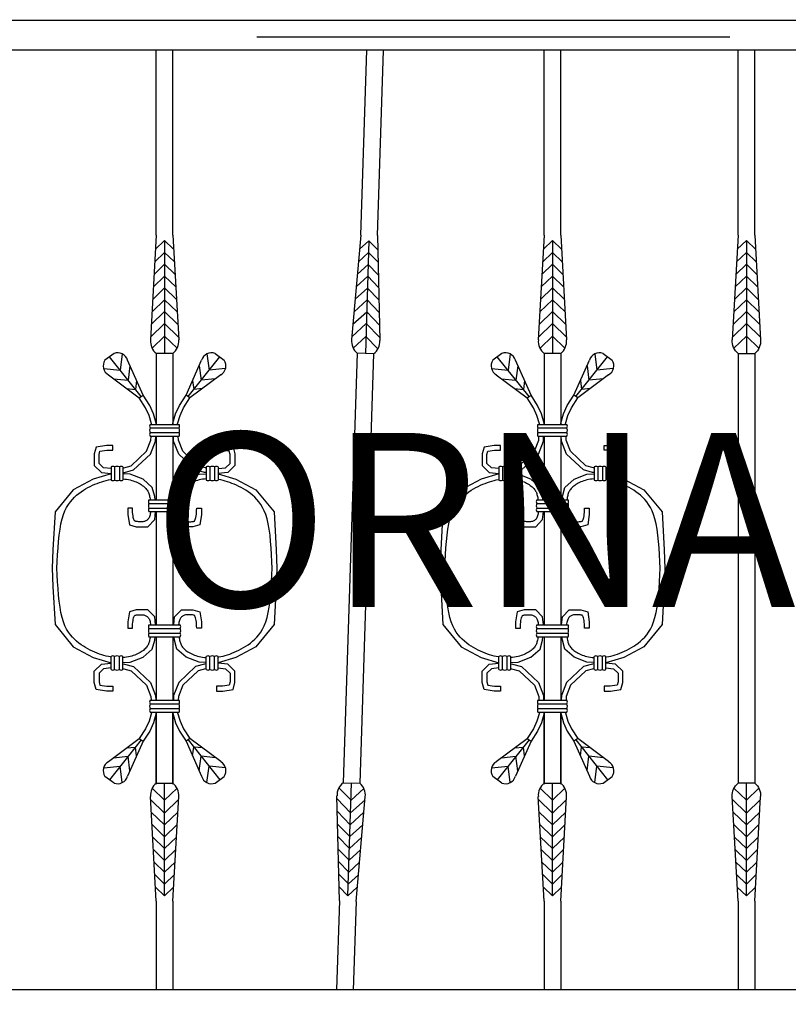
# Model space of a CAD drawing. Units: inches. Extents: x 2278 to 7495, y -71 to 1198.
# Tile 21 of 44: x 5033 to 5060, y 126 to 160. Entities that reach past the tile are written whole.
import ezdxf

# ---------------------------------------------------------------- set-up
doc = ezdxf.new("R2010")
doc.units = ezdxf.units.IN
doc.header["$MEASUREMENT"] = 0
doc.layers.add('A-ANNO-DIMS', color=2, linetype='Continuous', lineweight=18)
doc.layers.add('A-ELEV', color=7, linetype='Continuous', lineweight=25)
doc.styles.get("Standard").update_dxf_attribs({"font": 'arial.ttf'})
doc.dimstyles.get("Standard").update_dxf_attribs({"dimtxt": 6, "dimasz": 3, "dimexe": 0.18, "dimexo": 0.0625, "dimgap": 0.09, "dimtad": 0, "dimtih": 1, "dimtoh": 1, "dimdec": 0, "dimzin": 0, "dimdsep": 46, "dimlunit": 3, "dimtxsty": 'Standard', "dimblk": 'ARCHTICK', "dimcen": 0.09, "dimadec": 0, "dimazin": 0, "dimtfac": 1, "dimtdec": 0, "dimtofl": 0, "dimtmove": 0, "dimatfit": 3, "dimfxl": 1, "dimtolj": 1, "dimtzin": 0, "dimarcsym": 0})

# ---------------------------------------------------------------- blocks, each defined once
blk = doc.blocks.new('BALUSTER-ORNATE-A')
for p, q in [((3.585, 26.003), (3.585, 32.384)), ((4.155, 26.003), (4.155, 32.38)), ((3.585, 26.003), (3.383, 22.393)), ((3.558, 25.516), (3.87, 25.818)), ((3.87, 25.818), (3.87, 21.929)), ((4.182, 25.516), (3.87, 25.818)), ((4.155, 26.003), (4.357, 22.393)), ((3.533, 25.084), (3.87, 25.41)), ((4.207, 25.084), (3.87, 25.41)), ((3.509, 24.653), (3.87, 25.001)), ((4.231, 24.653), (3.87, 25.001)), ((3.485, 24.221), (3.87, 24.593)), ((4.255, 24.221), (3.87, 24.593)), ((3.461, 23.79), (3.87, 24.185)), ((4.279, 23.79), (3.87, 24.185)), ((3.437, 23.358), (3.87, 23.777)), ((4.303, 23.358), (3.87, 23.777)), ((3.413, 22.927), (3.87, 23.369)), ((4.327, 22.927), (3.87, 23.369)), ((3.388, 22.495), (3.87, 22.961)), ((4.352, 22.495), (3.87, 22.961)), ((3.442, 22.106), (3.87, 22.52)), ((4.299, 22.106), (3.87, 22.52)), ((2.128, 21.929), (1.813, 21.699)), ((3.063, 20.442), (1.97, 21.814)), ((2.412, 21.914), (2.339, 21.352)), ((3.585, 21.929), (3.585, 19.485)), ((4.155, 21.929), (3.585, 21.929)), ((4.155, 21.929), (4.155, 19.485)), ((4.677, 20.442), (5.77, 21.814)), ((5.328, 21.914), (5.401, 21.352)), ((5.612, 21.929), (5.927, 21.699)), ((1.774, 21.406), (2.339, 21.352)), ((3.131, 20.487), (2.594, 21.696)), ((2.678, 21.507), (2.613, 21.007)), ((4.609, 20.487), (5.146, 21.696)), ((5.062, 21.507), (5.127, 21.007)), ((5.966, 21.406), (5.401, 21.352)), ((1.936, 21.192), (2.995, 20.398)), ((2.111, 21.055), (2.613, 21.007)), ((5.804, 21.192), (4.745, 20.398)), ((5.629, 21.055), (5.127, 21.007)), ((2.562, 20.717), (2.868, 20.688)), ((2.907, 20.992), (2.868, 20.688)), ((4.833, 20.992), (4.872, 20.688)), ((5.178, 20.717), (4.872, 20.688)), ((2.995, 20.398), (3.131, 20.487)), ((3.217, 20.057), (2.995, 20.398)), ((3.36, 20.135), (3.131, 20.487)), ((4.38, 20.135), (4.609, 20.487)), ((4.523, 20.057), (4.745, 20.398)), ((4.745, 20.398), (4.609, 20.487)), ((3.337, 19.795), (3.217, 20.057)), ((3.49, 19.852), (3.36, 20.135)), ((4.25, 19.852), (4.38, 20.135)), ((4.403, 19.795), (4.523, 20.057)), ((3.421, 19.506), (3.337, 19.795)), ((3.585, 19.526), (3.49, 19.852)), ((4.155, 19.526), (4.25, 19.852)), ((4.319, 19.506), (4.403, 19.795)), ((3.37, 19.485), (4.37, 19.485)), ((3.37, 19.363), (4.37, 19.363)), ((3.42, 19.485), (3.421, 19.506)), ((3.583, 19.485), (3.585, 19.526)), ((4.157, 19.485), (4.155, 19.526)), ((4.32, 19.485), (4.319, 19.506)), ((3.37, 19.2), (4.37, 19.2)), ((3.37, 19.077), (4.37, 19.077)), ((3.396, 18.942), (3.402, 19.077)), ((3.558, 18.908), (3.565, 19.077)), ((3.585, 19.077), (3.585, 16.887)), ((4.155, 19.077), (4.155, 16.887)), ((4.182, 18.908), (4.175, 19.077)), ((4.344, 18.942), (4.338, 19.077)), ((1.513, 18.705), (1.449, 18.469)), ((1.866, 18.759), (1.513, 18.705)), ((2.084, 18.759), (1.866, 18.759)), ((2.084, 18.596), (2.084, 18.759)), ((3.247, 18.557), (3.396, 18.942)), ((3.385, 18.463), (3.558, 18.908)), ((4.355, 18.463), (4.182, 18.908)), ((4.493, 18.557), (4.344, 18.942)), ((5.656, 18.596), (5.656, 18.759)), ((5.656, 18.759), (5.874, 18.759)), ((5.874, 18.759), (6.227, 18.705)), ((6.227, 18.705), (6.291, 18.469)), ((1.449, 18.469), (1.449, 18.069)), ((1.612, 18.447), (1.642, 18.56)), ((1.612, 18.138), (1.612, 18.447)), ((1.642, 18.56), (1.879, 18.596)), ((1.879, 18.596), (2.084, 18.596)), ((2.719, 18.062), (3.247, 18.557)), ((2.801, 17.915), (3.385, 18.463)), ((4.939, 17.915), (4.355, 18.463)), ((5.021, 18.062), (4.493, 18.557)), ((5.861, 18.596), (5.656, 18.596)), ((6.098, 18.56), (5.861, 18.596)), ((6.128, 18.447), (6.098, 18.56)), ((6.128, 18.138), (6.128, 18.447)), ((6.291, 18.469), (6.291, 18.069)), ((1.449, 18.069), (1.694, 17.833)), ((1.767, 17.989), (1.612, 18.138)), ((2.026, 17.961), (1.767, 17.989)), ((2.026, 18.021), (2.026, 17.565)), ((2.148, 18.021), (2.148, 17.565)), ((2.311, 18.021), (2.311, 17.565)), ((2.434, 18.021), (2.434, 17.565)), ((2.434, 17.99), (2.462, 17.993)), ((2.462, 17.993), (2.719, 18.062)), ((5.278, 17.993), (5.021, 18.062)), ((5.306, 17.99), (5.278, 17.993)), ((5.306, 18.021), (5.306, 17.565)), ((5.429, 18.021), (5.429, 17.565)), ((5.592, 18.021), (5.592, 17.565)), ((5.714, 18.021), (5.714, 17.565)), ((5.714, 17.961), (5.973, 17.989)), ((5.973, 17.989), (6.128, 18.138)), ((6.291, 18.069), (6.046, 17.833)), ((2.026, 17.782), (1.412, 17.603)), ((1.694, 17.833), (2.026, 17.797)), ((2.434, 17.826), (2.492, 17.833)), ((2.683, 17.766), (2.434, 17.777)), ((2.492, 17.833), (2.801, 17.915)), ((3.128, 17.594), (2.683, 17.766)), ((4.612, 17.594), (5.057, 17.766)), ((5.248, 17.833), (4.939, 17.915)), ((5.057, 17.766), (5.306, 17.777)), ((5.306, 17.826), (5.248, 17.833)), ((6.046, 17.833), (5.714, 17.797)), ((5.714, 17.782), (6.328, 17.603)), ((1.412, 17.603), (0.722, 17.231)), ((1.15, 17.265), (1.23, 17.309)), ((1.23, 17.309), (1.309, 17.35)), ((1.309, 17.35), (1.389, 17.388)), ((1.389, 17.388), (1.469, 17.422)), ((1.469, 17.422), (1.549, 17.454)), ((1.549, 17.454), (1.627, 17.484)), ((1.627, 17.484), (1.705, 17.51)), ((1.705, 17.51), (1.782, 17.533)), ((1.782, 17.533), (1.858, 17.553)), ((1.858, 17.553), (1.933, 17.571)), ((1.933, 17.571), (2.007, 17.585)), ((2.007, 17.585), (2.026, 17.587)), ((2.434, 17.606), (2.499, 17.6)), ((2.499, 17.6), (2.563, 17.592)), ((2.563, 17.592), (2.624, 17.582)), ((2.624, 17.582), (2.683, 17.57)), ((2.683, 17.57), (2.739, 17.556)), ((2.739, 17.556), (2.792, 17.54)), ((2.792, 17.54), (2.843, 17.522)), ((2.843, 17.522), (2.891, 17.503)), ((2.891, 17.503), (2.937, 17.482)), ((2.937, 17.482), (2.981, 17.46)), ((2.981, 17.46), (3.024, 17.436)), ((3.024, 17.436), (3.064, 17.41)), ((3.064, 17.41), (3.102, 17.384)), ((3.102, 17.384), (3.138, 17.357)), ((3.446, 17.313), (3.128, 17.594)), ((3.138, 17.357), (3.171, 17.329)), ((3.171, 17.329), (3.201, 17.301)), ((3.201, 17.301), (3.228, 17.272)), ((3.528, 17.004), (3.446, 17.313)), ((4.212, 17.004), (4.294, 17.313)), ((4.294, 17.313), (4.612, 17.594)), ((4.539, 17.301), (4.512, 17.272)), ((4.569, 17.329), (4.539, 17.301)), ((4.602, 17.357), (4.569, 17.329)), ((4.638, 17.384), (4.602, 17.357)), ((4.676, 17.41), (4.638, 17.384)), ((4.716, 17.436), (4.676, 17.41)), ((4.759, 17.46), (4.716, 17.436)), ((4.803, 17.482), (4.759, 17.46)), ((4.849, 17.503), (4.803, 17.482)), ((4.897, 17.522), (4.849, 17.503)), ((4.948, 17.54), (4.897, 17.522)), ((5.001, 17.556), (4.948, 17.54)), ((5.057, 17.57), (5.001, 17.556)), ((5.116, 17.582), (5.057, 17.57)), ((5.177, 17.592), (5.116, 17.582)), ((5.241, 17.6), (5.177, 17.592)), ((5.306, 17.606), (5.241, 17.6)), ((5.733, 17.585), (5.714, 17.587)), ((5.807, 17.571), (5.733, 17.585)), ((5.882, 17.553), (5.807, 17.571)), ((5.958, 17.533), (5.882, 17.553)), ((6.035, 17.51), (5.958, 17.533)), ((6.113, 17.484), (6.035, 17.51)), ((6.191, 17.454), (6.113, 17.484)), ((6.271, 17.422), (6.191, 17.454)), ((6.351, 17.388), (6.271, 17.422)), ((6.328, 17.603), (7.018, 17.231)), ((6.431, 17.35), (6.351, 17.388)), ((6.51, 17.309), (6.431, 17.35)), ((6.59, 17.265), (6.51, 17.309)), ((0.722, 17.231), (0.096, 16.469)), ((0.692, 16.9), (0.764, 16.975)), ((0.764, 16.975), (0.839, 17.043)), ((0.839, 17.043), (0.916, 17.105)), ((0.916, 17.105), (0.993, 17.163)), ((0.993, 17.163), (1.071, 17.216)), ((1.071, 17.216), (1.15, 17.265)), ((3.228, 17.272), (3.252, 17.244)), ((3.252, 17.244), (3.272, 17.217)), ((3.272, 17.217), (3.288, 17.19)), ((3.288, 17.19), (3.303, 17.162)), ((3.303, 17.162), (3.316, 17.134)), ((3.316, 17.134), (3.327, 17.104)), ((3.327, 17.104), (3.337, 17.072)), ((3.337, 17.072), (3.346, 17.038)), ((3.346, 17.038), (3.354, 17.001)), ((3.354, 17.001), (3.361, 16.962)), ((3.361, 16.962), (3.368, 16.922)), ((3.542, 16.887), (3.528, 17.004)), ((4.198, 16.887), (4.212, 17.004)), ((4.379, 16.962), (4.372, 16.922)), ((4.386, 17.001), (4.379, 16.962)), ((4.394, 17.038), (4.386, 17.001)), ((4.403, 17.072), (4.394, 17.038)), ((4.413, 17.104), (4.403, 17.072)), ((4.424, 17.134), (4.413, 17.104)), ((4.437, 17.162), (4.424, 17.134)), ((4.452, 17.19), (4.437, 17.162)), ((4.468, 17.217), (4.452, 17.19)), ((4.489, 17.244), (4.468, 17.217)), ((4.512, 17.272), (4.489, 17.244)), ((6.669, 17.216), (6.59, 17.265)), ((6.747, 17.163), (6.669, 17.216)), ((6.824, 17.105), (6.747, 17.163)), ((6.901, 17.043), (6.824, 17.105)), ((6.976, 16.975), (6.901, 17.043)), ((7.048, 16.9), (6.976, 16.975)), ((7.018, 17.231), (7.644, 16.469)), ((0.438, 16.508), (0.495, 16.624)), ((0.495, 16.624), (0.557, 16.727)), ((0.557, 16.727), (0.623, 16.819)), ((0.623, 16.819), (0.692, 16.9)), ((3.329, 16.887), (4.411, 16.887)), ((3.329, 16.764), (4.411, 16.764)), ((3.368, 16.922), (3.374, 16.887)), ((4.372, 16.922), (4.366, 16.887)), ((7.117, 16.819), (7.048, 16.9)), ((7.183, 16.727), (7.117, 16.819)), ((7.245, 16.624), (7.183, 16.727)), ((7.302, 16.508), (7.245, 16.624)), ((0.096, 16.469), (0.025, 15.162)), ((0.34, 16.227), (0.386, 16.376)), ((0.386, 16.376), (0.438, 16.508)), ((2.764, 16.599), (2.602, 16.596)), ((2.602, 16.596), (2.602, 16.378)), ((2.602, 16.378), (2.656, 16.024)), ((2.766, 16.522), (2.764, 16.599)), ((2.769, 16.452), (2.766, 16.522)), ((2.775, 16.388), (2.769, 16.452)), ((2.783, 16.331), (2.775, 16.388)), ((2.792, 16.28), (2.783, 16.331)), ((3.329, 16.601), (4.411, 16.601)), ((3.329, 16.479), (4.411, 16.479)), ((3.346, 16.299), (3.333, 16.271)), ((3.357, 16.329), (3.346, 16.299)), ((3.368, 16.364), (3.357, 16.329)), ((3.376, 16.401), (3.368, 16.364)), ((3.383, 16.441), (3.376, 16.401)), ((3.388, 16.479), (3.383, 16.441)), ((3.528, 16.206), (3.557, 16.479)), ((3.585, 16.479), (3.585, 12.578)), ((4.155, 16.479), (4.155, 12.578)), ((4.212, 16.206), (4.183, 16.479)), ((4.352, 16.479), (4.357, 16.441)), ((4.357, 16.441), (4.364, 16.401)), ((4.364, 16.401), (4.372, 16.364)), ((4.372, 16.364), (4.383, 16.329)), ((4.383, 16.329), (4.394, 16.299)), ((4.394, 16.299), (4.407, 16.271)), ((4.948, 16.28), (4.957, 16.331)), ((4.957, 16.331), (4.965, 16.388)), ((4.965, 16.388), (4.971, 16.452)), ((4.971, 16.452), (4.974, 16.522)), ((4.974, 16.522), (4.976, 16.599)), ((4.976, 16.599), (5.138, 16.596)), ((5.138, 16.378), (5.084, 16.024)), ((5.138, 16.596), (5.138, 16.378)), ((7.354, 16.376), (7.302, 16.508)), ((7.4, 16.227), (7.354, 16.376)), ((7.644, 16.469), (7.715, 15.162)), ((0.267, 15.87), (0.3, 16.057)), ((0.3, 16.057), (0.34, 16.227)), ((2.656, 16.024), (2.892, 15.961)), ((2.803, 16.237), (2.792, 16.28)), ((2.815, 16.203), (2.803, 16.237)), ((2.825, 16.18), (2.815, 16.203)), ((2.834, 16.166), (2.825, 16.18)), ((2.84, 16.159), (2.834, 16.166)), ((2.846, 16.154), (2.84, 16.159)), ((2.852, 16.151), (2.846, 16.154)), ((2.863, 16.146), (2.852, 16.151)), ((2.88, 16.142), (2.863, 16.146)), ((2.905, 16.137), (2.88, 16.142)), ((2.892, 15.961), (3.292, 15.961)), ((2.936, 16.134), (2.905, 16.137)), ((2.971, 16.131), (2.936, 16.134)), ((3.008, 16.129), (2.971, 16.131)), ((3.045, 16.129), (3.008, 16.129)), ((3.081, 16.13), (3.045, 16.129)), ((3.117, 16.133), (3.081, 16.13)), ((3.15, 16.138), (3.117, 16.133)), ((3.179, 16.145), (3.15, 16.138)), ((3.205, 16.154), (3.179, 16.145)), ((3.228, 16.164), (3.205, 16.154)), ((3.249, 16.176), (3.228, 16.164)), ((3.268, 16.19), (3.249, 16.176)), ((3.286, 16.207), (3.268, 16.19)), ((3.303, 16.225), (3.286, 16.207)), ((3.292, 15.961), (3.528, 16.206)), ((3.318, 16.247), (3.303, 16.225)), ((3.333, 16.271), (3.318, 16.247)), ((4.448, 15.961), (4.212, 16.206)), ((4.407, 16.271), (4.422, 16.247)), ((4.422, 16.247), (4.437, 16.225)), ((4.437, 16.225), (4.454, 16.207)), ((4.848, 15.961), (4.448, 15.961)), ((4.454, 16.207), (4.472, 16.19)), ((4.472, 16.19), (4.491, 16.176)), ((4.491, 16.176), (4.512, 16.164)), ((4.512, 16.164), (4.535, 16.154)), ((4.535, 16.154), (4.561, 16.145)), ((4.561, 16.145), (4.59, 16.138)), ((4.59, 16.138), (4.623, 16.133)), ((4.623, 16.133), (4.659, 16.13)), ((4.659, 16.13), (4.695, 16.129)), ((4.695, 16.129), (4.732, 16.129)), ((4.732, 16.129), (4.769, 16.131)), ((4.769, 16.131), (4.804, 16.134)), ((4.804, 16.134), (4.835, 16.137)), ((4.835, 16.137), (4.86, 16.142)), ((5.084, 16.024), (4.848, 15.961)), ((4.86, 16.142), (4.877, 16.146)), ((4.877, 16.146), (4.888, 16.151)), ((4.888, 16.151), (4.895, 16.154)), ((4.895, 16.154), (4.9, 16.159)), ((4.9, 16.159), (4.906, 16.166)), ((4.906, 16.166), (4.915, 16.18)), ((4.915, 16.18), (4.925, 16.203)), ((4.925, 16.203), (4.937, 16.237)), ((4.937, 16.237), (4.948, 16.28)), ((7.44, 16.057), (7.4, 16.227)), ((7.473, 15.87), (7.44, 16.057)), ((0.217, 15.452), (0.239, 15.667)), ((0.239, 15.667), (0.267, 15.87)), ((7.501, 15.667), (7.473, 15.87)), ((7.523, 15.452), (7.501, 15.667)), ((0.199, 15.227), (0.217, 15.452)), ((7.541, 15.227), (7.523, 15.452)), ((0.025, 15.162), (0, 14.529)), ((0.173, 14.759), (0.185, 14.995)), ((0.185, 14.995), (0.199, 15.227)), ((7.555, 14.995), (7.541, 15.227)), ((7.567, 14.759), (7.555, 14.995)), ((7.715, 15.162), (7.74, 14.529)), ((0.163, 14.522), (0.173, 14.759)), ((7.577, 14.522), (7.567, 14.759)), ((0, 14.529), (0.025, 13.895)), ((0.173, 14.298), (0.163, 14.536)), ((0.185, 14.062), (0.173, 14.298)), ((7.555, 14.062), (7.567, 14.298)), ((7.567, 14.298), (7.577, 14.536)), ((7.74, 14.529), (7.715, 13.895)), ((0.199, 13.831), (0.185, 14.062)), ((7.541, 13.831), (7.555, 14.062)), ((0.025, 13.895), (0.096, 12.589)), ((0.217, 13.606), (0.199, 13.831)), ((0.239, 13.391), (0.217, 13.606)), ((7.501, 13.391), (7.523, 13.606)), ((7.523, 13.606), (7.541, 13.831)), ((7.715, 13.895), (7.644, 12.589)), ((0.267, 13.188), (0.239, 13.391)), ((7.473, 13.188), (7.501, 13.391)), ((0.3, 13), (0.267, 13.188)), ((0.34, 12.831), (0.3, 13)), ((2.656, 13.033), (2.602, 12.679)), ((2.892, 13.097), (2.656, 13.033)), ((2.825, 12.878), (2.834, 12.892)), ((2.834, 12.892), (2.84, 12.899)), ((2.84, 12.899), (2.846, 12.903)), ((2.846, 12.903), (2.852, 12.907)), ((2.852, 12.907), (2.863, 12.911)), ((2.863, 12.911), (2.88, 12.916)), ((2.88, 12.916), (2.905, 12.92)), ((3.292, 13.097), (2.892, 13.097)), ((2.905, 12.92), (2.936, 12.924)), ((2.936, 12.924), (2.971, 12.927)), ((2.971, 12.927), (3.008, 12.929)), ((3.008, 12.929), (3.045, 12.929)), ((3.045, 12.929), (3.081, 12.928)), ((3.081, 12.928), (3.117, 12.924)), ((3.117, 12.924), (3.15, 12.919)), ((3.15, 12.919), (3.179, 12.912)), ((3.179, 12.912), (3.205, 12.904)), ((3.205, 12.904), (3.228, 12.893)), ((3.228, 12.893), (3.249, 12.881)), ((3.528, 12.852), (3.292, 13.097)), ((4.212, 12.852), (4.448, 13.097)), ((4.448, 13.097), (4.848, 13.097)), ((4.512, 12.893), (4.491, 12.881)), ((4.535, 12.904), (4.512, 12.893)), ((4.561, 12.912), (4.535, 12.904)), ((4.59, 12.919), (4.561, 12.912)), ((4.623, 12.924), (4.59, 12.919)), ((4.659, 12.928), (4.623, 12.924)), ((4.695, 12.929), (4.659, 12.928)), ((4.732, 12.929), (4.695, 12.929)), ((4.769, 12.927), (4.732, 12.929)), ((4.804, 12.924), (4.769, 12.927)), ((4.835, 12.92), (4.804, 12.924)), ((4.86, 12.916), (4.835, 12.92)), ((4.848, 13.097), (5.084, 13.033)), ((4.877, 12.911), (4.86, 12.916)), ((4.888, 12.907), (4.877, 12.911)), ((4.895, 12.903), (4.888, 12.907)), ((4.9, 12.899), (4.895, 12.903)), ((4.906, 12.892), (4.9, 12.899)), ((4.915, 12.878), (4.906, 12.892)), ((5.084, 13.033), (5.138, 12.679)), ((7.4, 12.831), (7.44, 13)), ((7.44, 13), (7.473, 13.188)), ((0.096, 12.589), (0.722, 11.827)), ((0.386, 12.681), (0.34, 12.831)), ((0.438, 12.549), (0.386, 12.681)), ((2.602, 12.679), (2.602, 12.462)), ((2.766, 12.536), (2.769, 12.605)), ((2.769, 12.605), (2.775, 12.669)), ((2.775, 12.669), (2.783, 12.727)), ((2.783, 12.727), (2.792, 12.778)), ((2.792, 12.778), (2.803, 12.82)), ((2.803, 12.82), (2.815, 12.854)), ((2.815, 12.854), (2.825, 12.878)), ((3.249, 12.881), (3.268, 12.867)), ((3.268, 12.867), (3.286, 12.851)), ((3.286, 12.851), (3.303, 12.832)), ((3.303, 12.832), (3.318, 12.811)), ((3.318, 12.811), (3.333, 12.786)), ((3.329, 12.578), (4.411, 12.578)), ((3.333, 12.786), (3.346, 12.759)), ((3.346, 12.759), (3.357, 12.728)), ((3.357, 12.728), (3.368, 12.694)), ((3.368, 12.694), (3.376, 12.656)), ((3.376, 12.656), (3.383, 12.616)), ((3.383, 12.616), (3.388, 12.578)), ((3.557, 12.578), (3.528, 12.852)), ((4.183, 12.578), (4.212, 12.852)), ((4.357, 12.616), (4.352, 12.578)), ((4.364, 12.656), (4.357, 12.616)), ((4.372, 12.694), (4.364, 12.656)), ((4.383, 12.728), (4.372, 12.694)), ((4.394, 12.759), (4.383, 12.728)), ((4.407, 12.786), (4.394, 12.759)), ((4.422, 12.811), (4.407, 12.786)), ((4.437, 12.832), (4.422, 12.811)), ((4.454, 12.851), (4.437, 12.832)), ((4.472, 12.867), (4.454, 12.851)), ((4.491, 12.881), (4.472, 12.867)), ((4.925, 12.854), (4.915, 12.878)), ((4.937, 12.82), (4.925, 12.854)), ((4.948, 12.778), (4.937, 12.82)), ((4.957, 12.727), (4.948, 12.778)), ((4.965, 12.669), (4.957, 12.727)), ((4.971, 12.605), (4.965, 12.669)), ((4.974, 12.536), (4.971, 12.605)), ((5.138, 12.679), (5.138, 12.462)), ((7.644, 12.589), (7.018, 11.827)), ((7.302, 12.549), (7.354, 12.681)), ((7.354, 12.681), (7.4, 12.831)), ((0.495, 12.433), (0.438, 12.549)), ((0.557, 12.33), (0.495, 12.433)), ((0.623, 12.239), (0.557, 12.33)), ((0.692, 12.157), (0.623, 12.239)), ((2.602, 12.462), (2.764, 12.459)), ((2.764, 12.459), (2.766, 12.536)), ((3.329, 12.456), (4.411, 12.456)), ((3.329, 12.293), (4.411, 12.293)), ((4.976, 12.459), (4.974, 12.536)), ((5.138, 12.462), (4.976, 12.459)), ((7.048, 12.157), (7.117, 12.239)), ((7.117, 12.239), (7.183, 12.33)), ((7.183, 12.33), (7.245, 12.433)), ((7.245, 12.433), (7.302, 12.549)), ((0.764, 12.083), (0.692, 12.157)), ((0.839, 12.015), (0.764, 12.083)), ((0.916, 11.952), (0.839, 12.015)), ((0.993, 11.894), (0.916, 11.952)), ((1.071, 11.841), (0.993, 11.894)), ((3.303, 11.895), (3.288, 11.868)), ((3.316, 11.924), (3.303, 11.895)), ((3.327, 11.954), (3.316, 11.924)), ((3.337, 11.986), (3.327, 11.954)), ((3.329, 12.171), (4.411, 12.171)), ((3.346, 12.02), (3.337, 11.986)), ((3.354, 12.056), (3.346, 12.02)), ((3.361, 12.095), (3.354, 12.056)), ((3.368, 12.136), (3.361, 12.095)), ((3.374, 12.171), (3.368, 12.136)), ((3.446, 11.745), (3.528, 12.053)), ((3.528, 12.053), (3.542, 12.171)), ((3.585, 12.171), (3.585, 9.98)), ((4.155, 12.171), (4.155, 9.98)), ((4.212, 12.053), (4.198, 12.171)), ((4.294, 11.745), (4.212, 12.053)), ((4.366, 12.171), (4.372, 12.136)), ((4.372, 12.136), (4.379, 12.095)), ((4.379, 12.095), (4.386, 12.056)), ((4.386, 12.056), (4.394, 12.02)), ((4.394, 12.02), (4.403, 11.986)), ((4.403, 11.986), (4.413, 11.954)), ((4.413, 11.954), (4.424, 11.924)), ((4.424, 11.924), (4.437, 11.895)), ((4.437, 11.895), (4.452, 11.868)), ((6.669, 11.841), (6.747, 11.894)), ((6.747, 11.894), (6.824, 11.952)), ((6.824, 11.952), (6.901, 12.015)), ((6.901, 12.015), (6.976, 12.083)), ((6.976, 12.083), (7.048, 12.157)), ((0.722, 11.827), (1.412, 11.455)), ((1.15, 11.793), (1.071, 11.841)), ((1.23, 11.748), (1.15, 11.793)), ((1.309, 11.708), (1.23, 11.748)), ((1.389, 11.67), (1.309, 11.708)), ((1.469, 11.635), (1.389, 11.67)), ((1.549, 11.603), (1.469, 11.635)), ((1.627, 11.574), (1.549, 11.603)), ((1.705, 11.548), (1.627, 11.574)), ((1.782, 11.524), (1.705, 11.548)), ((2.843, 11.535), (2.792, 11.518)), ((2.891, 11.555), (2.843, 11.535)), ((2.937, 11.576), (2.891, 11.555)), ((2.981, 11.598), (2.937, 11.576)), ((3.024, 11.622), (2.981, 11.598)), ((3.064, 11.647), (3.024, 11.622)), ((3.102, 11.673), (3.064, 11.647)), ((3.138, 11.701), (3.102, 11.673)), ((3.128, 11.464), (3.446, 11.745)), ((3.171, 11.729), (3.138, 11.701)), ((3.201, 11.757), (3.171, 11.729)), ((3.228, 11.785), (3.201, 11.757)), ((3.252, 11.813), (3.228, 11.785)), ((3.272, 11.841), (3.252, 11.813)), ((3.288, 11.868), (3.272, 11.841)), ((4.612, 11.464), (4.294, 11.745)), ((4.452, 11.868), (4.468, 11.841)), ((4.468, 11.841), (4.489, 11.813)), ((4.489, 11.813), (4.512, 11.785)), ((4.512, 11.785), (4.539, 11.757)), ((4.539, 11.757), (4.569, 11.729)), ((4.569, 11.729), (4.602, 11.701)), ((4.602, 11.701), (4.638, 11.673)), ((4.638, 11.673), (4.676, 11.647)), ((4.676, 11.647), (4.716, 11.622)), ((4.716, 11.622), (4.759, 11.598)), ((4.759, 11.598), (4.803, 11.576)), ((4.803, 11.576), (4.849, 11.555)), ((4.849, 11.555), (4.897, 11.535)), ((4.897, 11.535), (4.948, 11.518)), ((5.958, 11.524), (6.035, 11.548)), ((6.035, 11.548), (6.113, 11.574)), ((6.113, 11.574), (6.191, 11.603)), ((6.191, 11.603), (6.271, 11.635)), ((6.271, 11.635), (6.351, 11.67)), ((7.018, 11.827), (6.328, 11.455)), ((6.351, 11.67), (6.431, 11.708)), ((6.431, 11.708), (6.51, 11.748)), ((6.51, 11.748), (6.59, 11.793)), ((6.59, 11.793), (6.669, 11.841)), ((1.412, 11.455), (2.026, 11.276)), ((1.449, 10.988), (1.694, 11.225)), ((1.694, 11.225), (2.026, 11.261)), ((1.858, 11.504), (1.782, 11.524)), ((1.933, 11.487), (1.858, 11.504)), ((2.007, 11.473), (1.933, 11.487)), ((2.026, 11.47), (2.007, 11.473)), ((2.026, 11.037), (2.026, 11.493)), ((2.148, 11.037), (2.148, 11.493)), ((2.311, 11.037), (2.311, 11.493)), ((2.434, 11.037), (2.434, 11.493)), ((2.499, 11.457), (2.434, 11.451)), ((2.434, 11.28), (2.683, 11.291)), ((2.434, 11.232), (2.492, 11.225)), ((2.492, 11.225), (2.801, 11.143)), ((2.563, 11.465), (2.499, 11.457)), ((2.624, 11.476), (2.563, 11.465)), ((2.683, 11.488), (2.624, 11.476)), ((2.739, 11.502), (2.683, 11.488)), ((2.683, 11.291), (3.128, 11.464)), ((2.792, 11.518), (2.739, 11.502)), ((5.057, 11.291), (4.612, 11.464)), ((5.248, 11.225), (4.939, 11.143)), ((4.948, 11.518), (5.001, 11.502)), ((5.001, 11.502), (5.057, 11.488)), ((5.057, 11.488), (5.116, 11.476)), ((5.306, 11.28), (5.057, 11.291)), ((5.116, 11.476), (5.177, 11.465)), ((5.177, 11.465), (5.241, 11.457)), ((5.241, 11.457), (5.306, 11.451)), ((5.306, 11.232), (5.248, 11.225)), ((5.306, 11.037), (5.306, 11.493)), ((5.429, 11.037), (5.429, 11.493)), ((5.592, 11.037), (5.592, 11.493)), ((5.714, 11.037), (5.714, 11.493)), ((5.714, 11.47), (5.733, 11.473)), ((6.328, 11.455), (5.714, 11.276)), ((6.046, 11.225), (5.714, 11.261)), ((5.733, 11.473), (5.807, 11.487)), ((5.807, 11.487), (5.882, 11.504)), ((5.882, 11.504), (5.958, 11.524)), ((6.291, 10.988), (6.046, 11.225)), ((1.449, 10.589), (1.449, 10.988)), ((1.767, 11.069), (1.612, 10.919)), ((1.612, 10.919), (1.612, 10.611)), ((2.026, 11.097), (1.767, 11.069)), ((2.434, 11.067), (2.462, 11.064)), ((2.462, 11.064), (2.719, 10.996)), ((2.719, 10.996), (3.247, 10.501)), ((2.801, 11.143), (3.385, 10.594)), ((4.939, 11.143), (4.355, 10.594)), ((5.021, 10.996), (4.493, 10.501)), ((5.278, 11.064), (5.021, 10.996)), ((5.306, 11.067), (5.278, 11.064)), ((5.714, 11.097), (5.973, 11.069)), ((5.973, 11.069), (6.128, 10.919)), ((6.128, 10.919), (6.128, 10.611)), ((6.291, 10.589), (6.291, 10.988)), ((1.513, 10.353), (1.449, 10.589)), ((1.612, 10.611), (1.642, 10.498)), ((3.385, 10.594), (3.558, 10.149)), ((4.355, 10.594), (4.182, 10.149)), ((6.128, 10.611), (6.098, 10.498)), ((6.227, 10.353), (6.291, 10.589)), ((1.866, 10.298), (1.513, 10.353)), ((1.642, 10.498), (1.879, 10.461)), ((2.084, 10.298), (1.866, 10.298)), ((1.879, 10.461), (2.084, 10.461)), ((2.084, 10.461), (2.084, 10.298)), ((3.247, 10.501), (3.396, 10.115)), ((4.493, 10.501), (4.344, 10.115)), ((5.861, 10.461), (5.656, 10.461)), ((5.656, 10.461), (5.656, 10.298)), ((5.656, 10.298), (5.874, 10.298)), ((6.098, 10.498), (5.861, 10.461)), ((5.874, 10.298), (6.227, 10.353)), ((3.37, 9.98), (4.37, 9.98)), ((3.37, 9.858), (4.37, 9.858)), ((3.396, 10.115), (3.402, 9.98)), ((3.558, 10.149), (3.565, 9.98)), ((4.182, 10.149), (4.175, 9.98)), ((4.344, 10.115), (4.338, 9.98)), ((3.421, 9.552), (3.337, 9.262)), ((3.37, 9.695), (4.37, 9.695)), ((3.37, 9.573), (4.37, 9.573)), ((3.42, 9.573), (3.421, 9.552)), ((3.585, 9.532), (3.49, 9.205)), ((3.583, 9.573), (3.585, 9.532)), ((3.585, 9.573), (3.585, 7.095)), ((3.585, 7.095), (3.585, 9.573)), ((4.155, 9.573), (4.155, 7.095)), ((4.155, 7.095), (4.155, 9.573)), ((4.157, 9.573), (4.155, 9.532)), ((4.155, 9.532), (4.25, 9.205)), ((4.32, 9.573), (4.319, 9.552)), ((4.319, 9.552), (4.403, 9.262)), ((3.337, 9.262), (3.217, 9.001)), ((3.49, 9.205), (3.36, 8.922)), ((4.25, 9.205), (4.38, 8.922)), ((4.403, 9.262), (4.523, 9.001)), ((3.217, 9.001), (2.995, 8.66)), ((3.36, 8.922), (3.131, 8.571)), ((4.38, 8.922), (4.609, 8.571)), ((4.523, 9.001), (4.745, 8.66)), ((1.936, 7.866), (2.995, 8.66)), ((3.063, 8.615), (1.97, 7.244)), ((3.131, 8.571), (2.594, 7.362)), ((2.995, 8.66), (3.131, 8.571)), ((4.745, 8.66), (4.609, 8.571)), ((4.609, 8.571), (5.146, 7.362)), ((4.677, 8.615), (5.77, 7.244)), ((5.804, 7.866), (4.745, 8.66)), ((2.562, 8.34), (2.868, 8.37)), ((2.907, 8.066), (2.868, 8.37)), ((4.833, 8.066), (4.872, 8.37)), ((5.178, 8.34), (4.872, 8.37)), ((2.111, 8.002), (2.613, 8.051)), ((2.678, 7.551), (2.613, 8.051)), ((5.062, 7.551), (5.127, 8.051)), ((5.629, 8.002), (5.127, 8.051)), ((1.774, 7.651), (2.339, 7.706)), ((2.412, 7.143), (2.339, 7.706)), ((5.328, 7.143), (5.401, 7.706)), ((5.966, 7.651), (5.401, 7.706)), ((2.128, 7.128), (1.813, 7.359)), ((3.585, 7.128), (4.155, 7.128)), ((3.87, 3.24), (3.87, 7.128)), ((5.612, 7.128), (5.927, 7.359)), ((3.442, 6.952), (3.87, 6.538)), ((4.299, 6.952), (3.87, 6.538)), ((3.585, 3.055), (3.383, 6.664)), ((3.388, 6.562), (3.87, 6.097)), ((4.352, 6.562), (3.87, 6.097)), ((4.155, 3.055), (4.357, 6.664)), ((3.413, 6.131), (3.87, 5.689)), ((4.327, 6.131), (3.87, 5.689)), ((3.437, 5.699), (3.87, 5.28)), ((4.303, 5.699), (3.87, 5.28)), ((3.461, 5.268), (3.87, 4.872)), ((4.279, 5.268), (3.87, 4.872)), ((3.485, 4.836), (3.87, 4.464)), ((4.255, 4.836), (3.87, 4.464)), ((3.509, 4.405), (3.87, 4.056)), ((4.231, 4.405), (3.87, 4.056)), ((3.533, 3.973), (3.87, 3.648)), ((4.207, 3.973), (3.87, 3.648)), ((3.558, 3.542), (3.87, 3.24)), ((4.182, 3.542), (3.87, 3.24)), ((3.585, 3.055), (3.585, 0)), ((4.155, 3.055), (4.155, 0))]:
    blk.add_line(p, q)
for centre, radius, start, end in [((3.929, 22.355), 0.547, 176.0178, 231.0717), ((3.811, 22.355), 0.547, 308.9283, 3.9822), ((2.253, 21.595), 0.356, 16.4025, 110.5063), ((5.487, 21.595), 0.356, 69.4937, 163.5975), ((2.111, 21.502), 0.356, 146.575, 240.6788), ((5.629, 21.502), 0.356, 299.3212, 33.425), ((3.475, 19.424), 0.121, 149.7768, 210.2232), ((3.563, 19.281), 0.209, 157.1017, 202.8983), ((4.265, 19.424), 0.121, 329.7768, 30.2232), ((4.177, 19.281), 0.209, 337.1017, 22.8983), ((3.475, 19.139), 0.121, 149.7768, 210.2232), ((4.265, 19.139), 0.121, 329.7768, 30.2232), ((2.087, 17.916), 0.121, 59.7768, 120.2232), ((2.23, 17.828), 0.209, 67.1017, 112.8983), ((2.373, 17.916), 0.121, 59.7768, 120.2232), ((5.368, 17.916), 0.121, 59.7768, 120.2232), ((5.51, 17.828), 0.209, 67.1017, 112.8983), ((5.653, 17.916), 0.121, 59.7768, 120.2232), ((2.087, 17.67), 0.121, 239.7768, 300.2232), ((2.23, 17.758), 0.209, 247.1017, 292.8983), ((2.373, 17.67), 0.121, 239.7768, 300.2232), ((5.368, 17.67), 0.121, 239.7768, 300.2232), ((5.51, 17.758), 0.209, 247.1017, 292.8983), ((5.653, 17.67), 0.121, 239.7768, 300.2232), ((3.434, 16.825), 0.121, 149.7768, 210.2232), ((3.522, 16.683), 0.209, 157.1017, 202.8983), ((4.306, 16.825), 0.121, 329.7768, 30.2232), ((4.218, 16.683), 0.209, 337.1017, 22.8983), ((3.434, 16.54), 0.121, 149.7768, 210.2232), ((4.306, 16.54), 0.121, 329.7768, 30.2232), ((3.434, 12.517), 0.121, 149.7768, 210.2232), ((4.306, 12.517), 0.121, 329.7768, 30.2232), ((3.522, 12.375), 0.209, 157.1017, 202.8983), ((3.434, 12.232), 0.121, 149.7768, 210.2232), ((4.218, 12.375), 0.209, 337.1017, 22.8983), ((4.306, 12.232), 0.121, 329.7768, 30.2232), ((2.087, 11.388), 0.121, 59.7768, 120.2232), ((2.23, 11.3), 0.209, 67.1017, 112.8983), ((2.373, 11.388), 0.121, 59.7768, 120.2232), ((5.368, 11.388), 0.121, 59.7768, 120.2232), ((5.51, 11.3), 0.209, 67.1017, 112.8983), ((5.653, 11.388), 0.121, 59.7768, 120.2232), ((2.087, 11.142), 0.121, 239.7768, 300.2232), ((2.23, 11.23), 0.209, 247.1017, 292.8983), ((2.373, 11.142), 0.121, 239.7768, 300.2232), ((5.368, 11.142), 0.121, 239.7768, 300.2232), ((5.51, 11.23), 0.209, 247.1017, 292.8983), ((5.653, 11.142), 0.121, 239.7768, 300.2232), ((3.475, 9.919), 0.121, 149.7768, 210.2232), ((3.563, 9.776), 0.209, 157.1017, 202.8983), ((4.265, 9.919), 0.121, 329.7768, 30.2232), ((4.177, 9.776), 0.209, 337.1017, 22.8983), ((3.475, 9.634), 0.121, 149.7768, 210.2232), ((4.265, 9.634), 0.121, 329.7768, 30.2232), ((2.111, 7.555), 0.356, 119.3212, 213.425), ((5.629, 7.555), 0.356, 326.575, 60.6788), ((2.253, 7.462), 0.356, 249.4937, 343.5975), ((3.929, 6.703), 0.547, 128.9283, 183.9822), ((3.811, 6.703), 0.547, 356.0178, 51.0717), ((5.487, 7.462), 0.356, 196.4025, 290.5063)]:
    blk.add_arc(centre, radius, start, end)
blk = doc.blocks.new('RAIL-BAR-A')
for p, q in [((0.202, 26.003), (0.202, 32.38)), ((0.773, 26.003), (0.773, 32.38)), ((0.202, 26.003), (0, 22.393)), ((0.175, 25.516), (0.488, 25.818)), ((0.488, 25.818), (0.488, 21.929)), ((0.8, 25.516), (0.488, 25.818)), ((0.773, 26.003), (0.975, 22.393)), ((0.151, 25.084), (0.488, 25.41)), ((0.824, 25.084), (0.488, 25.41)), ((0.127, 24.653), (0.488, 25.001)), ((0.848, 24.653), (0.488, 25.001)), ((0.103, 24.221), (0.488, 24.593)), ((0.873, 24.221), (0.488, 24.593)), ((0.079, 23.79), (0.488, 24.185)), ((0.897, 23.79), (0.488, 24.185)), ((0.054, 23.358), (0.488, 23.777)), ((0.921, 23.358), (0.488, 23.777)), ((0.03, 22.927), (0.488, 23.369)), ((0.945, 22.927), (0.488, 23.369)), ((0.006, 22.495), (0.488, 22.961)), ((0.969, 22.495), (0.488, 22.961)), ((0.059, 22.106), (0.488, 22.52)), ((0.916, 22.106), (0.488, 22.52)), ((0.202, 21.929), (0.202, 7.128)), ((0.773, 21.929), (0.202, 21.929)), ((0.773, 21.929), (0.773, 7.128)), ((0.202, 7.128), (0.773, 7.128)), ((0.488, 3.24), (0.488, 7.128)), ((0.059, 6.952), (0.488, 6.538)), ((0.916, 6.952), (0.488, 6.538)), ((0.202, 3.055), (0, 6.664)), ((0.006, 6.562), (0.488, 6.097)), ((0.969, 6.562), (0.488, 6.097)), ((0.773, 3.055), (0.975, 6.664)), ((0.03, 6.131), (0.488, 5.689)), ((0.945, 6.131), (0.488, 5.689)), ((0.054, 5.699), (0.488, 5.28)), ((0.921, 5.699), (0.488, 5.28)), ((0.079, 5.268), (0.488, 4.872)), ((0.897, 5.268), (0.488, 4.872)), ((0.103, 4.836), (0.488, 4.464)), ((0.873, 4.836), (0.488, 4.464)), ((0.127, 4.405), (0.488, 4.056)), ((0.848, 4.405), (0.488, 4.056)), ((0.151, 3.973), (0.488, 3.648)), ((0.824, 3.973), (0.488, 3.648)), ((0.175, 3.542), (0.488, 3.24)), ((0.8, 3.542), (0.488, 3.24)), ((0.202, 3.055), (0.202, 0)), ((0.773, 3.055), (0.773, 0))]:
    blk.add_line(p, q)
for centre, start, end in [((0.546, 22.355), 176.0178, 231.0717), ((0.429, 22.355), 308.9283, 3.9822), ((0.546, 6.703), 128.9283, 183.9822), ((0.429, 6.703), 356.0178, 51.0717)]:
    blk.add_arc(centre, 0.547, start, end)
blk = doc.blocks.new('RAIL-BAR-B')
for p, q in [((17.353, 32.832), (1.059, 32.832)), ((0.203, 26.003), (0.203, 32.38)), ((0.773, 26.003), (0.773, 32.38)), ((0.203, 26.003), (0.001, 22.393)), ((0.176, 25.516), (0.488, 25.818)), ((0.488, 25.818), (0.488, 21.929)), ((0.801, 25.516), (0.488, 25.818)), ((0.773, 26.003), (0.976, 22.393)), ((0.152, 25.084), (0.488, 25.41)), ((0.825, 25.084), (0.488, 25.41)), ((0.128, 24.653), (0.488, 25.001)), ((0.849, 24.653), (0.488, 25.001)), ((0.103, 24.221), (0.488, 24.593)), ((0.873, 24.221), (0.488, 24.593)), ((0.079, 23.79), (0.488, 24.185)), ((0.897, 23.79), (0.488, 24.185)), ((0.055, 23.358), (0.488, 23.777)), ((0.922, 23.358), (0.488, 23.777)), ((0.031, 22.927), (0.488, 23.369)), ((0.946, 22.927), (0.488, 23.369)), ((0.007, 22.495), (0.488, 22.961)), ((0.97, 22.495), (0.488, 22.961)), ((0.06, 22.106), (0.488, 22.52)), ((0.917, 22.106), (0.488, 22.52)), ((0.203, 21.929), (0.203, 7.128)), ((0.773, 21.929), (0.203, 21.929)), ((0.773, 21.929), (0.773, 7.128)), ((0.203, 7.128), (0.773, 7.128)), ((0.488, 3.24), (0.488, 7.128)), ((0.06, 6.952), (0.488, 6.538)), ((0.917, 6.952), (0.488, 6.538)), ((0.203, 3.055), (0.001, 6.664)), ((0.007, 6.562), (0.488, 6.097)), ((0.97, 6.562), (0.488, 6.097)), ((0.773, 3.055), (0.976, 6.664)), ((0.031, 6.131), (0.488, 5.689)), ((0.946, 6.131), (0.488, 5.689)), ((0.055, 5.699), (0.488, 5.28)), ((0.922, 5.699), (0.488, 5.28)), ((0.079, 5.268), (0.488, 4.872)), ((0.897, 5.268), (0.488, 4.872)), ((0.103, 4.836), (0.488, 4.464)), ((0.873, 4.836), (0.488, 4.464)), ((0.128, 4.405), (0.488, 4.056)), ((0.849, 4.405), (0.488, 4.056)), ((0.152, 3.973), (0.488, 3.648)), ((0.825, 3.973), (0.488, 3.648)), ((0.176, 3.542), (0.488, 3.24)), ((0.801, 3.542), (0.488, 3.24)), ((0.203, 3.055), (0.203, 0)), ((0.773, 3.055), (0.773, 0))]:
    blk.add_line(p, q)
for centre, start, end in [((0.547, 22.355), 176.0178, 231.0717), ((0.429, 22.355), 308.9283, 3.9822), ((0.547, 6.703), 128.9283, 183.9822), ((0.429, 6.703), 356.0178, 51.0717)]:
    blk.add_arc(centre, 0.547, start, end)
blk = doc.blocks.new('_ArchTick')
at = {"color": 0, "linetype": 'ByBlock', "const_width": 0.15}
blk.add_lwpolyline([(-0.5, -0.5), (0.5, 0.5)], dxfattribs=at)
blk = doc.blocks.new('*D59')
at = {"layer": 'A-ANNO-DIMS', "color": 0, "lineweight": -2, "transparency": 16777216}
for p, q in [((5096.589, 159.183), (5101.564, 159.183)), ((5101.384, 159.183), (5101.384, 146.185)), ((5101.384, 126.799), (5101.384, 139.796)), ((5096.589, 126.799), (5101.564, 126.799))]:
    blk.add_line(p, q, dxfattribs=at)
at = {"layer": 'Defpoints', "color": 0, "transparency": 16777216}
for p in [(5096.527, 159.183), (5101.384, 159.183), (5096.527, 126.799)]:
    blk.add_point(p, dxfattribs=at)
at = {"layer": 'A-ANNO-DIMS', "color": 0, "lineweight": -2, "transparency": 16777216, "xscale": 3, "yscale": 3, "zscale": 3}
for p, rotation in [((5101.384, 159.183), 90), ((5101.384, 126.799), 270)]:
    blk.add_blockref('_ArchTick', p, dxfattribs=dict(at, rotation=rotation))
at = {"layer": 'A-ANNO-DIMS', "color": 0, "transparency": 16777216, "insert": (5101.384, 142.991), "char_height": 6, "attachment_point": 5}
blk.add_mtext('\\A1;ORNATE BALUSTER 2\'-8 1/2" TYP.', dxfattribs=at)
blk = doc.blocks.new('*D123')
at = {"layer": 'A-ANNO-DIMS', "color": 0, "lineweight": -2, "transparency": 16777216}
for p, q in [((4736.95, 340.157), (4736.95, -23.427)), ((5145.676, -1.81), (5145.676, -23.427)), ((4736.95, -23.247), (4923.929, -23.247)), ((5145.676, -23.247), (4958.697, -23.247))]:
    blk.add_line(p, q, dxfattribs=at)
at = {"layer": 'Defpoints', "color": 0, "transparency": 16777216}
for p in [(4736.95, 340.219), (5145.676, -1.747), (5145.676, -23.247)]:
    blk.add_point(p, dxfattribs=at)
at = {"layer": 'A-ANNO-DIMS', "color": 0, "lineweight": -2, "transparency": 16777216, "xscale": 3, "yscale": 3, "zscale": 3, "rotation": 180}
blk.add_blockref('_ArchTick', (4736.95, -23.247), dxfattribs=at)
at = {"layer": 'A-ANNO-DIMS', "color": 0, "lineweight": -2, "transparency": 16777216, "xscale": 3, "yscale": 3, "zscale": 3}
blk.add_blockref('_ArchTick', (5145.676, -23.247), dxfattribs=at)
at = {"layer": 'A-ANNO-DIMS', "color": 0, "transparency": 16777216, "insert": (4941.313, -23.247), "char_height": 6, "attachment_point": 5}
blk.add_mtext('\\A1;34\'-0 1/2"', dxfattribs=at)
blk = doc.blocks.new('*D130')
at = {"layer": 'A-ANNO-DIMS', "color": 0, "lineweight": -2, "transparency": 16777216}
for p, q in [((5016.176, 99.315), (5016.176, 361.899)), ((5016.176, 361.719), (5048.095, 361.719)), ((5096.176, 361.719), (5064.257, 361.719)), ((5096.176, 99.315), (5096.176, 361.899))]:
    blk.add_line(p, q, dxfattribs=at)
at = {"layer": 'Defpoints', "color": 0, "transparency": 16777216}
for p in [(5096.176, 361.719), (5016.176, 99.253), (5096.176, 99.253)]:
    blk.add_point(p, dxfattribs=at)
at = {"layer": 'A-ANNO-DIMS', "color": 0, "lineweight": -2, "transparency": 16777216, "xscale": 3, "yscale": 3, "zscale": 3, "rotation": 180}
blk.add_blockref('_ArchTick', (5016.176, 361.719), dxfattribs=at)
at = {"layer": 'A-ANNO-DIMS', "color": 0, "lineweight": -2, "transparency": 16777216, "xscale": 3, "yscale": 3, "zscale": 3}
blk.add_blockref('_ArchTick', (5096.176, 361.719), dxfattribs=at)
at = {"layer": 'A-ANNO-DIMS', "color": 0, "transparency": 16777216, "insert": (5056.176, 361.719), "char_height": 6, "attachment_point": 5}
blk.add_mtext('\\A1;6\'-8"', dxfattribs=at)

msp = doc.modelspace()

# ---------------------------------------------------------------- linework, layer by layer
at = {"layer": 'A-ELEV'}
for p, q in [((5065.039, 160.198), (4971.673, 160.198)), ((5065.039, 159.179), (4971.673, 159.179)), ((5065.039, 126.799), (4971.673, 126.799))]:
    msp.add_line(p, q, dxfattribs=at)

# ---------------------------------------------------------------- block references
at = {"layer": 'A-ELEV', "extrusion": (0, 0, -1), "zscale": -1}
msp.add_blockref('RAIL-BAR-B', (-5058.928, 126.799), dxfattribs=at)
at = {"layer": 'A-ELEV'}
for p in [(5034.528, 126.799), (5047.889, 126.799)]:
    msp.add_blockref('BALUSTER-ORNATE-A', p, dxfattribs=at)
at = {"layer": 'A-ELEV', "rotation": 358.1636620689618}
msp.add_blockref('RAIL-BAR-A', (5044.123, 126.822), dxfattribs=at)

# ---------------------------------------------------------------- dimensions: what is measured, and where the dimension line sits
at = {"layer": 'A-ANNO-DIMS'}
for base, p1, p2, picture, middle in [((5096.176, 361.719), (5016.176, 99.253), (5096.176, 99.253), '*D130', (5056.176, 361.719)), ((5145.676, -23.247), (4736.95, 340.219), (5145.676, -1.747), '*D123', (4941.313, -23.247))]:
    dim = msp.add_linear_dim(base=base, p1=p1, p2=p2, dimstyle='Standard', override={"dimdec": 1, "dimlfac": 1, "dimrnd": 0, "dimzin": 1, "dimdsep": 46, "dimlunit": 4, "dimfrac": 2}, dxfattribs=at)
    dim.commit()
    dim.dimension.update_dxf_attribs({"geometry": picture, "text_midpoint": middle})
dim = msp.add_linear_dim(base=(5101.384, 159.183), p1=(5096.527, 126.799), p2=(5096.527, 159.183), angle=90, text='ORNATE BALUSTER <> TYP.', dimstyle='Standard', override={"dimdec": 1, "dimrnd": 0, "dimzin": 1, "dimlunit": 4, "dimfrac": 2}, dxfattribs=at)
dim.commit()
dim.dimension.update_dxf_attribs({"geometry": '*D59', "text_midpoint": (5101.384, 142.991)})

doc.saveas('drawing.dxf')
